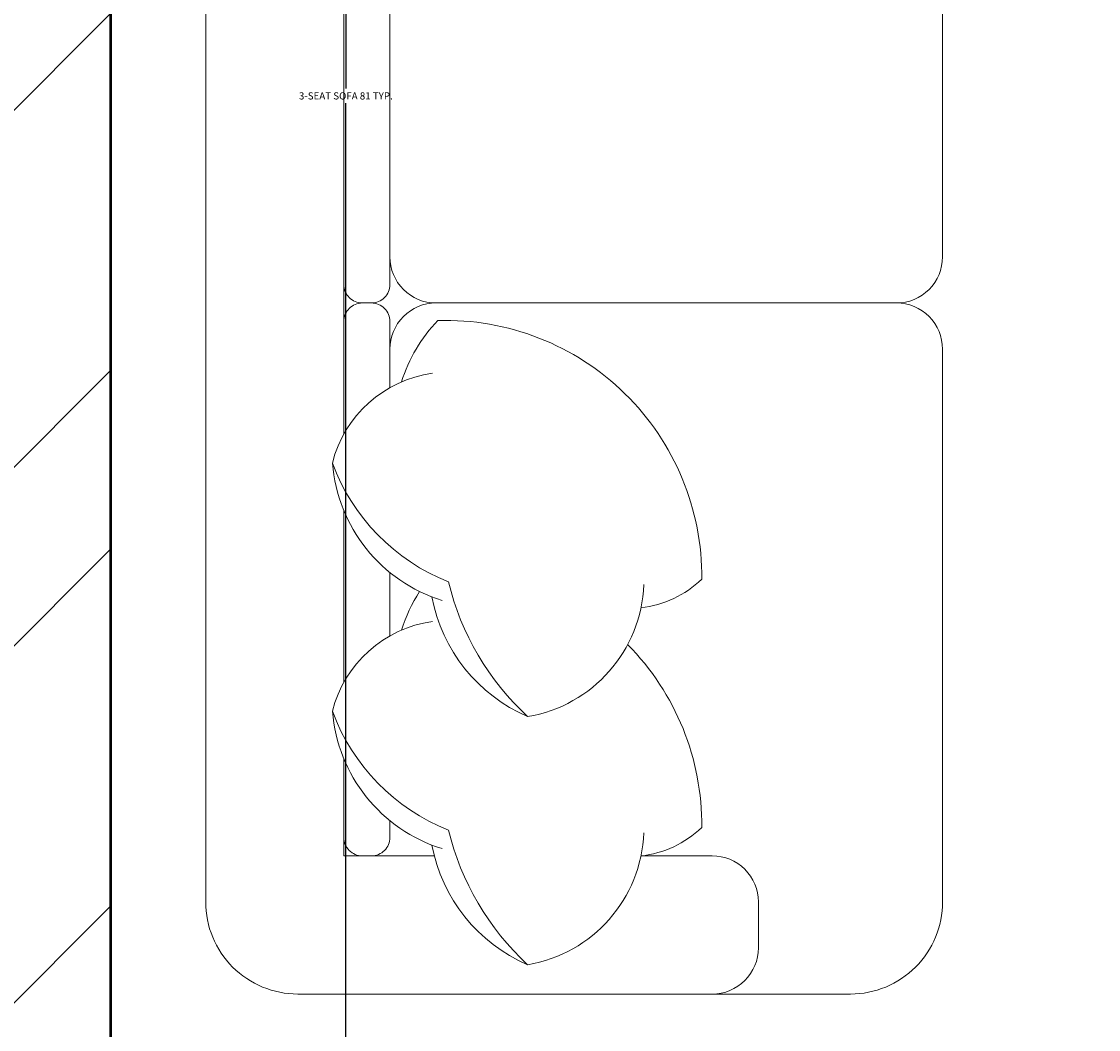
# Model space of a CAD drawing. Units: inches. Extents: x 963 to 2075, y 289 to 2657.
# Tile 50 of 98: x 1511 to 1538, y 1752 to 1778. Entities that reach past the tile are written whole.
import ezdxf

# ---------------------------------------------------------------- set-up
doc = ezdxf.new("R2010")
doc.units = ezdxf.units.IN
for name, color, linetype, lineweight in [('A-ANNO-DIMS', 2, 'Continuous', 18), ('A-FURN', 8, 'Continuous', 18), ('A-WALL', 7, 'Continuous', 50), ('A-WALL-PATT', 8, 'Continuous', 13)]:
    doc.layers.add(name, color=color, linetype=linetype, lineweight=lineweight)
doc.styles.get("Standard").update_dxf_attribs({"font": 'arial.ttf'})
doc.dimstyles.get("Standard").update_dxf_attribs({"dimtxt": 0.18, "dimasz": 0.18, "dimexe": 0.18, "dimexo": 0.0625, "dimgap": 0.09, "dimtad": 0, "dimtih": 1, "dimtoh": 1, "dimdec": 4, "dimzin": 0, "dimdsep": 46, "dimtxsty": 'Standard', "dimcen": 0.09, "dimadec": 0, "dimazin": 0, "dimtfac": 1, "dimtdec": 4, "dimtofl": 0, "dimtmove": 0, "dimatfit": 3, "dimfxl": 1, "dimtolj": 1, "dimtzin": 0, "dimarcsym": 0})

# ---------------------------------------------------------------- blocks, each defined once
blk = doc.blocks.new('*D28')
at = {"layer": 'A-ANNO-DIMS', "color": 0, "lineweight": -2, "transparency": 16777216}
for p, q in [((1506.727, 1816.319), (1519.012, 1816.319)), ((1518.832, 1816.139), (1518.832, 1775.944)), ((1518.832, 1735.382), (1518.832, 1775.577)), ((1506.727, 1735.202), (1519.012, 1735.202))]:
    blk.add_line(p, q, dxfattribs=at)
at = {"layer": 'A-ANNO-DIMS', "color": 0, "transparency": 16777216}
for points in [[(1518.802, 1816.139), (1518.862, 1816.139), (1518.832, 1816.319)], [(1518.802, 1735.382), (1518.862, 1735.382), (1518.832, 1735.202)]]:
    blk.add_solid(points, dxfattribs=at)
at = {"layer": 'Defpoints', "color": 0, "transparency": 16777216}
for p in [(1506.665, 1816.319), (1518.832, 1816.319), (1506.665, 1735.202)]:
    blk.add_point(p, dxfattribs=at)
at = {"layer": 'A-ANNO-DIMS', "color": 0, "transparency": 16777216, "insert": (1518.832, 1775.761), "char_height": 0.18, "attachment_point": 5}
blk.add_mtext('\\A1;3-SEAT SOFA 81 TYP.', dxfattribs=at)

msp = doc.modelspace()

# ---------------------------------------------------------------- hatches: boundary and pattern name
at = {"layer": 'A-WALL-PATT'}
h = msp.add_hatch(dxfattribs=at)
h.set_pattern_fill('ANSI32', color=256)
h.paths.add_polyline_path([(1473.609, 2163.068), (1473.609, 2165.318), (1376.422, 2165.318), (1376.422, 2227.983), (1371.922, 2227.983), (1371.922, 2214.818), (1368.405, 2214.818), (1368.405, 2210.318), (1371.922, 2210.318), (1371.922, 2160.818), (1395.922, 2160.818), (1395.922, 2090.318), (1217.345, 2090.318), (1217.345, 2085.818), (1395.922, 2085.818), (1458.922, 2085.818), (1458.922, 2108.318), (1454.422, 2108.318), (1454.422, 2090.318), (1400.422, 2090.318), (1400.422, 2160.818), (1473.609, 2160.818)])
h.paths.add_polyline_path([(1649.422, 2210.318), (1653.225, 2210.318), (1653.225, 2214.818), (1649.422, 2214.818), (1649.422, 2227.983), (1644.922, 2227.983), (1644.922, 2165.318), (1550.099, 2165.318), (1550.099, 2160.818), (1620.922, 2160.818), (1620.922, 2112.818), (1555.446, 2112.818), (1555.446, 2108.318), (1584.327, 2108.318), (1584.327, 2084.916), (1588.827, 2084.916), (1588.827, 2108.318), (1625.422, 2108.318), (1667.951, 2108.318), (1667.951, 2022.667), (1588.827, 2022.667), (1588.827, 2047.408), (1584.327, 2047.408), (1584.327, 1996.003), (1588.827, 1996.003), (1588.827, 2018.318), (1667.951, 2018.167), (1667.951, 1928.318), (1625.422, 1928.318), (1625.422, 1923.818), (1672.451, 1923.818), (1672.451, 1928.318), (1672.451, 1946.663), (1785.446, 1946.663), (1785.446, 1951.163), (1743.034, 1951.163), (1743.034, 2017.922), (1841.422, 2017.922), (1841.422, 2014.775), (1845.922, 2014.775), (1845.922, 2017.922), (1905.922, 2017.922), (1905.922, 1987.511), (1910.422, 1987.511), (1910.422, 2022.422), (1910.422, 2068.517), (1905.922, 2068.517), (1905.922, 2022.422), (1845.922, 2022.422), (1845.922, 2025.851), (1843.672, 2025.851), (1841.422, 2025.851), (1841.422, 2022.422), (1743.034, 2022.422), (1743.034, 2084.031), (1768.451, 2084.031), (1785.446, 2084.031), (1785.446, 2088.531), (1672.451, 2088.531), (1672.451, 2112.818), (1667.951, 2112.818), (1625.422, 2112.818), (1625.422, 2160.818), (1649.422, 2160.818)])
h.paths.add_polyline_path([(1672.451, 2084.031), (1738.534, 2084.031), (1738.534, 1951.163), (1672.451, 1951.163)], flags=16)
h.paths.add_polyline_path([(1672.451, 2084.031), (1738.534, 2084.031), (1705.492, 2017.597)], flags=0)
h.paths.add_polyline_path([(1262.766, 2085.818), (1258.266, 2085.818), (1258.266, 2023.278), (1184.422, 2023.278), (1184.422, 2018.778), (1258.266, 2018.778), (1258.266, 1950.818), (1262.766, 1950.818)])
h.paths.add_polyline_path([(1312.266, 2085.818), (1307.766, 2085.818), (1307.766, 1950.818), (1312.266, 1950.818)])
h.paths.add_polyline_path([(1458.922, 1950.818), (1395.922, 1950.818), (1216.568, 1950.818), (1216.568, 1946.318), (1346.422, 1946.318), (1395.922, 1946.318), (1395.922, 1875.818), (1371.922, 1875.818), (1371.922, 1826.318), (1368.931, 1826.318), (1368.931, 1821.818), (1371.922, 1821.818), (1371.922, 1813.622), (1376.422, 1813.622), (1376.422, 1871.318), (1474.504, 1871.318), (1474.504, 1873.568), (1474.504, 1875.818), (1400.422, 1875.818), (1400.422, 1946.318), (1454.422, 1946.318), (1454.422, 1928.318), (1458.922, 1928.318)])
h.paths.add_polyline_path([(1184.422, 2120.778), (1167.922, 2120.778), (1167.922, 2134.812), (1165.672, 2134.812), (1163.422, 2134.812), (1163.422, 2120.778), (1119.922, 2120.778), (1119.922, 2098.095), (1124.422, 2098.095), (1124.422, 2116.278), (1167.922, 2116.278), (1179.922, 2116.278), (1179.922, 2045.916), (1184.422, 2045.916), (1184.422, 2090.318), (1184.422, 2116.278)])
h.paths.add_polyline_path([(1124.422, 2018.778), (1179.922, 2018.778), (1179.922, 2016.294), (1184.422, 2016.294), (1184.422, 2023.278), (1184.422, 2026.588), (1182.172, 2026.588), (1179.922, 2026.588), (1179.922, 2023.278), (1124.422, 2023.278), (1124.422, 2074.095), (1119.922, 2074.095), (1119.922, 2018.778), (1119.922, 1979.633), (1124.422, 1979.633)])
h.paths.add_polyline_path([(1184.422, 1925.778), (1184.422, 1946.318), (1184.422, 1996.073), (1182.172, 1996.073), (1179.922, 1996.073), (1179.922, 1925.778), (1124.422, 1925.778), (1124.422, 1955.633), (1119.922, 1955.502), (1119.922, 1921.278), (1158.922, 1921.278), (1158.922, 1909.983), (1163.422, 1909.983), (1163.422, 1921.278), (1184.422, 1921.278)])
h.paths.add_polyline_path([(1341.449, 1826.318), (1163.422, 1826.318), (1163.422, 1849.983), (1158.922, 1849.983), (1158.922, 1821.818), (1158.922, 1804.033), (1163.422, 1804.033), (1163.422, 1821.818), (1341.449, 1821.818)])
h.paths.add_polyline_path([(1222.981, 1713.818), (1163.422, 1713.818), (1163.422, 1744.033), (1161.172, 1744.033), (1158.922, 1744.033), (1158.922, 1713.818), (1119.922, 1713.818), (1119.922, 1694.65), (1124.422, 1694.65), (1124.422, 1709.318), (1158.922, 1709.318), (1222.981, 1709.318)])
h.paths.add_polyline_path([(1328.422, 1713.818), (1252.042, 1713.818), (1252.042, 1711.568), (1252.042, 1709.318), (1256.422, 1709.318), (1256.422, 1547.318), (1232.937, 1547.318), (1232.937, 1545.068), (1232.937, 1542.818), (1292.422, 1542.818), (1292.422, 1527.634), (1296.922, 1527.634), (1296.922, 1542.818), (1299.464, 1542.818), (1299.464, 1547.318), (1260.922, 1547.318), (1260.922, 1658.318), (1343.661, 1658.318), (1343.661, 1660.568), (1343.661, 1662.818), (1328.422, 1662.818), (1328.422, 1676.589), (1327.402, 1676.589), (1323.922, 1676.589), (1323.922, 1662.818), (1260.922, 1662.818), (1260.922, 1709.318), (1323.922, 1709.318), (1323.922, 1699.851), (1328.422, 1699.851)])
h.paths.add_polyline_path([(1649.422, 1875.818), (1625.422, 1875.818), (1625.422, 1928.318), (1620.922, 1928.318), (1588.827, 1928.318), (1588.827, 1950.59), (1584.327, 1950.59), (1584.327, 1928.318), (1555.446, 1928.318), (1555.446, 1923.818), (1620.922, 1923.818), (1620.922, 1875.818), (1548.952, 1875.818), (1548.952, 1873.568), (1548.952, 1871.318), (1644.922, 1871.318), (1644.922, 1813.622), (1649.422, 1813.622), (1649.422, 1821.818), (1652.045, 1821.818), (1652.045, 1824.068), (1652.045, 1826.318), (1649.422, 1826.318)])
h.paths.add_polyline_path([(1512.922, 1871.318), (1516.476, 1871.318), (1516.476, 1875.818), (1512.922, 1875.818), (1512.922, 1923.818), (1512.922, 1928.318), (1512.922, 1930.827), (1508.422, 1930.827), (1508.422, 1875.818), (1504.411, 1875.818), (1504.411, 1871.318), (1508.422, 1871.318), (1508.422, 1713.818), (1376.422, 1713.818), (1376.422, 1743.325), (1371.922, 1743.325), (1371.922, 1709.318), (1371.922, 1706.01), (1376.422, 1706.01), (1376.422, 1709.318), (1508.422, 1709.318), (1508.422, 1547.318), (1501.871, 1547.318), (1501.871, 1542.818), (1508.422, 1542.818), (1508.422, 1482.818), (1508.422, 1436.318), (1512.922, 1436.318), (1512.922, 1542.818), (1519.318, 1542.818), (1519.318, 1545.068), (1519.318, 1547.318), (1512.922, 1547.318), (1512.922, 1709.318), (1644.922, 1709.318), (1644.922, 1707.548), (1649.422, 1707.548), (1649.422, 1709.318), (1649.422, 1743.325), (1644.922, 1743.325), (1644.922, 1713.818), (1512.922, 1713.818)])
h.paths.add_polyline_path([(1129.884, 1545.068), (1129.884, 1547.318), (1124.422, 1547.318), (1095.922, 1547.318), (1095.922, 1614.818), (1124.422, 1614.818), (1124.422, 1619.318), (1095.922, 1619.318), (1091.422, 1619.318), (1091.422, 1542.818), (1095.922, 1542.818), (1119.922, 1542.818), (1129.884, 1542.818)])
h.paths.add_polyline_path([(1208.422, 1542.818), (1211.74, 1542.818), (1211.74, 1547.318), (1198.851, 1547.318), (1198.851, 1542.818), (1203.922, 1542.818), (1203.922, 1478.318), (1208.422, 1478.318), (1296.922, 1478.318), (1296.922, 1503.634), (1292.422, 1503.634), (1292.422, 1482.818), (1208.422, 1482.818)])
h.paths.add_polyline_path([(1430.422, 1542.818), (1435.699, 1542.818), (1435.699, 1545.068), (1435.699, 1547.318), (1422.658, 1547.318), (1422.658, 1545.068), (1422.658, 1542.818), (1425.922, 1542.818), (1425.922, 1482.857), (1341.922, 1482.857), (1341.922, 1502.732), (1337.422, 1502.732), (1337.422, 1478.357), (1425.922, 1478.357), (1425.922, 1440.818), (1425.922, 1436.318), (1430.422, 1436.318)])
h.paths.add_polyline_path([(1698.482, 2004.259), (1727.695, 2004.259), (1727.695, 2022.916), (1698.482, 2022.916)], flags=8)

# ---------------------------------------------------------------- linework, layer by layer
at = {"layer": 'A-FURN', "ltscale": 0.03}
msp.add_lwpolyline([(1531.529, 1801.839, -0.414214), (1533.846, 1799.522), (1533.846, 1785.616, -0.414214), (1532.687, 1784.457, -0.414214), (1533.846, 1783.298), (1533.846, 1771.71, -0.414214), (1532.687, 1770.552, -0.414214), (1533.846, 1769.393), (1533.846, 1755.487, -0.414214), (1531.529, 1753.169), (1517.623, 1753.169, -0.414214), (1515.305, 1755.487), (1515.305, 1799.522, -0.414214), (1517.623, 1801.839)], format="xyb", close=True, dxfattribs=at)
at = {"layer": 'A-FURN'}
for points in [[(1518.782, 1793.997), (1518.782, 1767.254)], [(1518.782, 1765.326), (1518.782, 1761.012)]]:
    msp.add_lwpolyline(points, dxfattribs=at)
msp.add_lwpolyline([(1518.782, 1771.015), (1518.782, 1783.994, -0.414214), (1519.245, 1784.457), (1519.477, 1784.457, -0.414214), (1519.941, 1783.994), (1519.941, 1771.015, -0.414214), (1519.477, 1770.552), (1519.245, 1770.552, -0.414214)], format="xyb", close=True, dxfattribs=at)
for points in [[(1519.941, 1771.71, 0.414214), (1521.099, 1770.552)], [(1518.782, 1767.254), (1518.782, 1770.088, -0.414214), (1519.245, 1770.552), (1519.477, 1770.552, -0.414214), (1519.941, 1770.088), (1519.941, 1768.421, -0.414214)], [(1519.941, 1769.393, -0.414214), (1521.099, 1770.552), (1532.687, 1770.552, -0.414214)], [(1526.256, 1762.886, 0.165541), (1527.787, 1763.603, 0.425989), (1521.149, 1770.111, 0.121523), (1520.234, 1768.566, -7.115464)], [(1521.256, 1763.068, -0.306663), (1518.494, 1766.525, -0.30633), (1521.016, 1768.783, 0.872847)], [(1523.406, 1760.149, -0.14773), (1521.415, 1763.536, -0.213343), (1518.494, 1766.525, -0.178662)], [(1518.782, 1761.012), (1518.782, 1765.326, -0.414214)], [(1519.941, 1763.773), (1519.941, 1762.178, -0.414214)], [(1520.687, 1763.295, 0.071865), (1520.234, 1762.323, -7.115464)], [(1526.327, 1763.47, -0.356772), (1523.406, 1760.149, -0.249542), (1520.999, 1763.158, 9.61688)], [(1521.256, 1756.826, -0.306663), (1518.494, 1760.282, -0.30633), (1521.016, 1762.54, 0.872847)], [(1526.256, 1756.643, 0.165541), (1527.787, 1757.36, 0.200231), (1525.923, 1761.96, 0.121523)], [(1523.406, 1753.907, -0.14773), (1521.415, 1757.294, -0.213343), (1518.494, 1760.282, -0.178662)], [(1518.782, 1759.084), (1518.782, 1756.646), (1521.059, 1756.646, -0.414214)], [(1518.782, 1757.109), (1518.782, 1759.084, -0.414214)], [(1519.941, 1757.53), (1519.941, 1757.109, -0.414214), (1519.477, 1756.646), (1519.245, 1756.646, -0.414214), (1518.782, 1757.109)], [(1526.327, 1757.227, -0.356772), (1523.406, 1753.907, -0.249542), (1520.999, 1756.916, 9.61688)], [(1526.257, 1756.646), (1528.052, 1756.646, -0.414214), (1529.211, 1755.487), (1529.211, 1754.328, -0.414214), (1528.052, 1753.169)]]:
    msp.add_lwpolyline(points, format="xyb", dxfattribs=at)
at = {"layer": 'A-WALL'}
msp.add_line((1512.922, 1713.818), (1512.922, 1871.318), dxfattribs=at)

# ---------------------------------------------------------------- dimensions: what is measured, and where the dimension line sits
at = {"layer": 'A-ANNO-DIMS'}
dim = msp.add_linear_dim(base=(1518.832, 1816.319), p1=(1506.665, 1735.202), p2=(1506.665, 1816.319), angle=90, text='3-SEAT SOFA <> TYP.', dimstyle='Standard', override={"dimdec": 0, "dimlfac": 1, "dimrnd": 0, "dimzin": 0, "dimdsep": 46, "dimlunit": 2}, dxfattribs=at)
dim.commit()
dim.dimension.update_dxf_attribs({"geometry": '*D28', "text_midpoint": (1518.832, 1775.761)})

doc.saveas('drawing.dxf')
